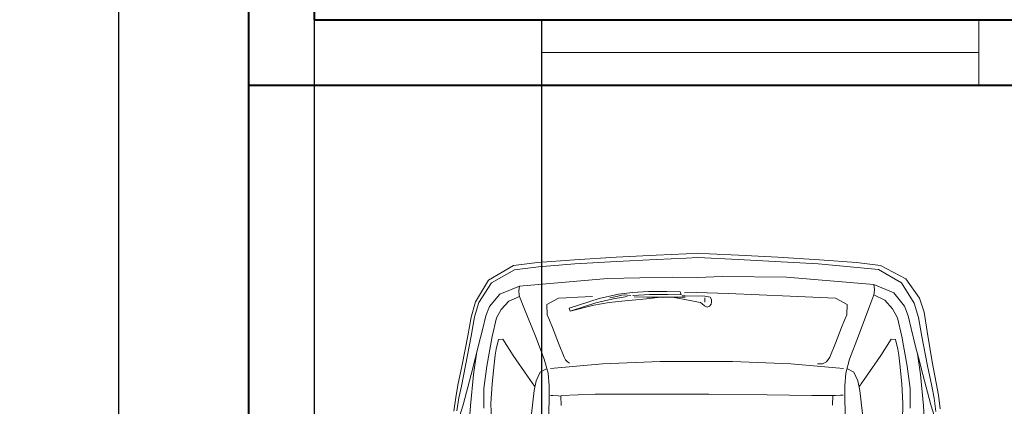
# Model space of a CAD drawing. Units: inches. Extents: x -19 to 419, y -828 to 43.
# Tile 3 of 9: x -9 to 126, y -627 to -574. Entities that reach past the tile are written whole.
import ezdxf

# ---------------------------------------------------------------- set-up
doc = ezdxf.new("R2010")
doc.units = ezdxf.units.IN
doc.header["$MEASUREMENT"] = 0
for name, color, linetype, lineweight in [('A-ANNO-DIMS', 2, 'Continuous', 18), ('A-EQPM-VEHI', 8, 'Continuous', 13), ('A-GLAZ', 4, 'Continuous', 20), ('A-WALL', 7, 'Continuous', 40)]:
    doc.layers.add(name, color=color, linetype=linetype, lineweight=lineweight)
doc.styles.get("Standard").update_dxf_attribs({"font": 'arial.ttf'})
doc.dimstyles.get("Standard").update_dxf_attribs({"dimtxt": 0.18, "dimasz": 0.18, "dimexe": 0.18, "dimexo": 0.0625, "dimgap": 0.09, "dimtad": 0, "dimtih": 1, "dimtoh": 1, "dimdec": 0, "dimzin": 0, "dimdsep": 46, "dimlunit": 3, "dimtxsty": 'Standard', "dimcen": 0.09, "dimadec": 0, "dimazin": 0, "dimtfac": 1, "dimtdec": 0, "dimtofl": 0, "dimtmove": 0, "dimatfit": 3, "dimfxl": 1, "dimtolj": 1, "dimtzin": 0, "dimarcsym": 0})

# ---------------------------------------------------------------- blocks, each defined once
blk = doc.blocks.new('*D2')
at = {"layer": 'A-ANNO-DIMS', "color": 0, "lineweight": -2, "transparency": 16777216}
for p, q in [((22.68, 4.77), (4.74, 4.77)), ((4.92, 4.59), (4.92, -387.33)), ((4.92, -785.55), (4.92, -393.64)), ((22.68, -785.73), (4.74, -785.73))]:
    blk.add_line(p, q, dxfattribs=at)
at = {"layer": 'A-ANNO-DIMS', "color": 0, "transparency": 16777216}
for points in [[(4.89, 4.59), (4.95, 4.59), (4.92, 4.77)], [(4.89, -785.55), (4.95, -785.55), (4.92, -785.73)]]:
    blk.add_solid(points, dxfattribs=at)
at = {"layer": 'Defpoints', "color": 0, "transparency": 16777216}
for p in [(22.74, 4.77), (4.92, -785.73), (22.74, -785.73)]:
    blk.add_point(p, dxfattribs=at)
at = {"layer": 'A-ANNO-DIMS', "color": 0, "transparency": 16777216, "insert": (4.92, -390.48), "char_height": 6, "attachment_point": 5}
blk.add_mtext('\\A1;65\'-11"', dxfattribs=at)
blk = doc.blocks.new('WIN-60X9')
for p, q in [((60, 9), (0, 9)), ((0, 9), (0, 0)), ((60, 0), (60, 9)), ((0, 4.5), (60, 4.5)), ((0, 0), (60, 0))]:
    blk.add_line(p, q)
blk = doc.blocks.new('*D49')
at = {"layer": 'A-ANNO-DIMS', "color": 0, "lineweight": -2, "transparency": 16777216}
for p, q in [((31.74, -574.3), (31.74, -827.51)), ((62.91, -574.3), (62.91, -827.51)), ((31.92, -827.33), (46.99, -827.33)), ((62.73, -827.33), (47.65, -827.33))]:
    blk.add_line(p, q, dxfattribs=at)
at = {"layer": 'A-ANNO-DIMS', "color": 0, "transparency": 16777216}
for points in [[(31.92, -827.3), (31.92, -827.36), (31.74, -827.33)], [(62.73, -827.3), (62.73, -827.36), (62.91, -827.33)]]:
    blk.add_solid(points, dxfattribs=at)
at = {"layer": 'Defpoints', "color": 0, "transparency": 16777216}
for p in [(31.74, -574.23), (62.91, -574.23), (62.91, -827.33)]:
    blk.add_point(p, dxfattribs=at)
at = {"layer": 'A-ANNO-DIMS', "color": 0, "transparency": 16777216, "insert": (47.32, -827.33), "char_height": 0.18, "attachment_point": 5}
blk.add_mtext('\\A1;2\'-7"', dxfattribs=at)

msp = doc.modelspace()

# ---------------------------------------------------------------- linework, layer by layer
at = {"layer": 'A-EQPM-VEHI'}
for p, q in [((73.18, -606.78), (78.63, -606.51)), ((78.63, -606.51), (82.76, -606.33)), ((82.76, -606.33), (84.39, -606.26)), ((84.39, -606.26), (85.95, -606.33)), ((85.95, -606.33), (89.95, -606.51)), ((89.95, -606.51), (95.33, -606.78)), ((59.08, -607.94), (62.39, -607.52)), ((62.39, -607.52), (67.44, -607.13)), ((67.51, -607.72), (62.49, -608.11)), ((67.44, -607.13), (73.18, -606.78)), ((73.21, -607.37), (67.51, -607.72)), ((78.65, -607.1), (73.21, -607.37)), ((82.75, -606.92), (78.65, -607.1)), ((84.37, -606.85), (82.75, -606.92)), ((89.88, -607.09), (84.37, -606.85)), ((100.89, -607.7), (89.88, -607.09)), ((95.33, -606.78), (101.07, -607.13)), ((109.15, -608.49), (100.89, -607.7)), ((101.07, -607.13), (106.12, -607.52)), ((106.12, -607.52), (109.43, -607.94)), ((55.65, -609.93), (59.08, -607.94)), ((59.2, -608.52), (56.05, -610.32)), ((62.49, -608.11), (59.2, -608.52)), ((112.31, -610.32), (109.15, -608.49)), ((109.43, -607.94), (112.9, -609.75)), ((53.85, -612.9), (55.65, -609.93)), ((56.05, -610.32), (54.33, -613.02)), ((59.89, -610.74), (71.96, -609.7)), ((71.96, -609.7), (80.85, -609.51)), ((80.85, -609.51), (84.32, -609.58)), ((84.32, -609.58), (87.73, -609.46)), ((87.73, -609.46), (96.52, -609.55)), ((96.52, -609.55), (108.53, -610.55)), ((111.26, -611.69), (108.53, -610.55)), ((108.59, -611.2), (108.53, -610.55)), ((114.06, -613.09), (112.31, -610.32)), ((112.9, -609.75), (114.79, -612.41)), ((55.79, -613.54), (57.19, -611.84)), ((57.19, -611.84), (59.89, -610.74)), ((59.83, -611.4), (59.89, -610.74)), ((59.86, -611.93), (59.83, -611.4)), ((73.49, -611.87), (70.84, -612.47)), ((75.39, -611.61), (73.49, -611.87)), ((77.61, -611.49), (75.39, -611.61)), ((75.52, -612.04), (77.74, -611.92)), ((80.12, -611.49), (77.61, -611.49)), ((77.74, -611.92), (80.25, -611.92)), ((81.94, -611.55), (80.12, -611.49)), ((80.25, -611.92), (82.07, -611.97)), ((82.07, -611.97), (81.94, -611.55)), ((82.54, -611.69), (84.25, -611.63)), ((84.25, -611.63), (88.54, -611.79)), ((88.54, -611.79), (97.05, -612.12)), ((108.53, -611.96), (108.56, -611.74)), ((108.56, -611.74), (108.59, -611.2)), ((112.7, -613.49), (111.26, -611.69)), ((53.26, -615), (53.85, -612.9)), ((54.33, -613.02), (53.73, -614.97)), ((57.4, -613.94), (58.44, -612.81)), ((58.44, -612.81), (59.89, -612.16)), ((59.89, -612.16), (59.86, -611.93)), ((60.61, -613.93), (59.89, -612.16)), ((63.64, -613.27), (65.24, -612.4)), ((65.24, -612.4), (66.32, -612.34)), ((66.32, -612.34), (67.92, -612.27)), ((70.84, -612.47), (66.71, -613.78)), ((66.84, -614.21), (70.39, -613.07)), ((67.92, -612.27), (69.91, -612.18)), ((70.1, -613.39), (72.22, -613.01)), ((70.39, -613.07), (72.75, -612.5)), ((72.22, -613.01), (73.93, -612.8)), ((72.29, -612.38), (73.23, -612.16)), ((72.75, -612.5), (74.69, -612.16)), ((73.23, -612.16), (73.96, -612.01)), ((73.93, -612.8), (75.37, -612.66)), ((73.96, -612.01), (74.25, -611.96)), ((74.25, -611.96), (75.19, -612.03)), ((75.37, -612.66), (77.32, -612.48)), ((75.44, -612.05), (75.47, -612.05)), ((75.47, -612.05), (75.5, -612.04)), ((75.5, -612.04), (75.52, -612.04)), ((75.65, -612.24), (77.36, -612.25)), ((77.32, -612.48), (79.27, -612.25)), ((77.36, -612.25), (80.62, -612.25)), ((80.62, -612.25), (82.63, -612.26)), ((80.89, -612.25), (83.31, -612.74)), ((82.23, -612.08), (82.61, -612.08)), ((82.61, -612.08), (85.31, -612.15)), ((83.31, -612.74), (84.44, -612.96)), ((84.44, -612.96), (84.73, -613.01)), ((84.96, -613.19), (84.73, -613.01)), ((85.28, -613.48), (84.96, -613.19)), ((85.31, -612.15), (86.07, -612.27)), ((85.35, -612.36), (85.31, -612.94)), ((86.19, -613.22), (85.96, -613.51)), ((86.07, -612.27), (86.24, -612.6)), ((86.25, -612.97), (86.19, -613.22)), ((86.24, -612.6), (86.25, -612.97)), ((97.05, -612.12), (103.27, -612.4)), ((103.27, -612.4), (104.87, -613.27)), ((107.84, -613.78), (108.53, -611.96)), ((110.01, -612.66), (108.53, -611.96)), ((111.08, -613.89), (110.01, -612.66)), ((114.66, -615.07), (114.06, -613.09)), ((114.79, -612.41), (115.42, -614.33)), ((55.28, -614.84), (55.79, -613.54)), ((56.76, -615.1), (57.4, -613.94)), ((62.08, -617.61), (60.61, -613.93)), ((63.69, -614.68), (63.64, -613.27)), ((66.71, -613.78), (66.84, -614.21)), ((66.84, -614.21), (70.1, -613.39)), ((85.63, -613.64), (85.28, -613.48)), ((85.96, -613.51), (85.63, -613.64)), ((104.87, -613.27), (104.81, -614.68)), ((106.4, -617.56), (107.84, -613.78)), ((111.74, -615.1), (111.08, -613.89)), ((113.22, -614.84), (112.7, -613.49)), ((115.42, -614.33), (115.83, -617)), ((52.8, -617.58), (53.26, -615)), ((53.73, -614.97), (53.28, -617.6)), ((54.86, -616.55), (55.28, -614.84)), ((56.14, -617.67), (56.76, -615.1)), ((64.02, -615.42), (63.69, -614.68)), ((64.41, -616.44), (64.02, -615.42)), ((104.49, -615.42), (104.1, -616.44)), ((104.81, -614.68), (104.49, -615.42)), ((112.37, -617.67), (111.74, -615.1)), ((113.65, -616.55), (113.22, -614.84)), ((115.11, -617.67), (114.66, -615.07)), ((54.25, -619.02), (54.86, -616.55)), ((65.24, -618.58), (64.41, -616.44)), ((104.1, -616.44), (103.27, -618.58)), ((114.25, -619.02), (113.65, -616.55)), ((115.83, -617), (116.52, -621.14)), ((52.04, -621.55), (52.8, -617.58)), ((53.28, -617.6), (52.51, -621.65)), ((55.43, -621.71), (56.14, -617.67)), ((56.68, -619.4), (57.02, -618.08)), ((57.02, -618.08), (57.6, -618.05)), ((57.6, -618.05), (59.04, -620.26)), ((63.31, -620.75), (62.08, -617.61)), ((66.01, -620.49), (65.24, -618.58)), ((103.27, -618.58), (102.49, -620.49)), ((105.19, -620.75), (106.4, -617.56)), ((110.91, -618.05), (109.46, -620.26)), ((111.49, -618.08), (110.91, -618.05)), ((111.83, -619.4), (111.49, -618.08)), ((113.07, -621.71), (112.37, -617.67)), ((115.88, -621.67), (115.11, -617.67)), ((53.87, -620.56), (54.25, -619.02)), ((56.57, -620.24), (56.68, -619.4)), ((111.94, -620.24), (111.83, -619.4)), ((114.63, -620.56), (114.25, -619.02)), ((53.28, -622.86), (53.87, -620.56)), ((53.58, -622.89), (54, -620.05)), ((56.43, -621.45), (56.57, -620.24)), ((59.04, -620.26), (60.99, -623.08)), ((63.82, -622.68), (63.31, -620.75)), ((66.22, -620.87), (66.01, -620.49)), ((66.47, -621.14), (66.22, -620.87)), ((66.76, -621.3), (66.47, -621.14)), ((71.31, -621.43), (79.19, -621.08)), ((79.19, -621.08), (84.12, -621.07)), ((84.12, -621.07), (89.13, -621.08)), ((89.13, -621.08), (97.13, -621.43)), ((102.03, -621.14), (101.45, -621.39)), ((102.49, -620.49), (102.03, -621.14)), ((104.68, -622.68), (105.19, -620.75)), ((109.46, -620.26), (107.52, -623.08)), ((112.07, -621.45), (111.94, -620.24)), ((114.93, -622.89), (114.51, -620.05)), ((115.22, -622.86), (114.63, -620.56)), ((116.52, -621.14), (117.06, -624.02)), ((51.46, -624.34), (52.04, -621.55)), ((52.51, -621.65), (51.93, -624.49)), ((55.03, -624.8), (55.43, -621.71)), ((56.17, -624.14), (56.43, -621.45)), ((62.2, -623.72), (62.72, -622.56)), ((62.72, -622.56), (63.7, -622.04)), ((63.96, -624.42), (63.82, -622.68)), ((64.15, -622.04), (71.31, -621.43)), ((97.13, -621.43), (104.36, -622.04)), ((101.45, -621.39), (100.8, -621.4)), ((104.55, -624.42), (104.68, -622.68)), ((105.79, -622.56), (104.81, -622.04)), ((106.31, -623.72), (105.79, -622.56)), ((112.34, -624.14), (112.07, -621.45)), ((113.48, -624.8), (113.07, -621.71)), ((116.47, -624.48), (115.88, -621.67)), ((52.17, -627.01), (53.28, -622.86)), ((53.18, -627.18), (53.58, -622.89)), ((60.99, -623.08), (61.96, -624.48)), ((61.9, -625.06), (62.2, -623.72)), ((106.61, -625.06), (106.31, -623.72)), ((107.52, -623.08), (106.54, -624.48)), ((115.32, -627.18), (114.93, -622.89)), ((116.34, -627.01), (115.22, -622.86)), ((117.06, -624.02), (117.37, -625.69)), ((51.15, -626.02), (51.46, -624.34)), ((51.93, -624.49), (51.59, -626.09)), ((55.01, -627.49), (55.03, -624.8)), ((55.99, -626.85), (56.17, -624.14)), ((61.53, -628.28), (61.9, -625.06)), ((63.96, -626.08), (63.96, -624.42)), ((104.55, -626.08), (104.55, -624.42)), ((106.97, -628.28), (106.61, -625.06)), ((112.51, -626.85), (112.34, -624.14)), ((113.5, -627.49), (113.48, -624.8)), ((116.77, -626.12), (116.47, -624.48)), ((50.91, -627.91), (51.15, -626.02)), ((51.59, -626.09), (51.31, -627.85)), ((63.86, -631.09), (63.96, -626.08)), ((64.49, -625.77), (64.16, -625.75)), ((65.19, -625.8), (64.49, -625.77)), ((65.57, -625.82), (65.19, -625.8)), ((65.61, -627.13), (65.57, -625.82)), ((65.63, -625.76), (70.28, -625.59)), ((70.28, -625.59), (77.53, -625.55)), ((77.53, -625.55), (85.88, -625.59)), ((85.88, -625.59), (93.87, -625.68)), ((93.87, -625.68), (100.03, -625.75)), ((100.03, -625.75), (102.88, -625.76)), ((102.84, -627.08), (102.88, -625.76)), ((102.88, -625.76), (103.26, -625.75)), ((103.26, -625.75), (103.96, -625.71)), ((103.96, -625.71), (104.29, -625.7)), ((104.65, -631.09), (104.55, -626.08)), ((117.01, -627.96), (116.77, -626.12)), ((117.37, -625.69), (117.61, -627.58)), ((51.11, -630.39), (52.17, -627.01)), ((52.97, -630.19), (53.18, -627.18)), ((56.07, -629.23), (55.99, -626.85)), ((112.44, -629.23), (112.51, -626.85)), ((115.53, -630.19), (115.32, -627.18)), ((117.4, -630.39), (116.34, -627.01))]:
    msp.add_line(p, q, dxfattribs=at)
at = {"layer": 'A-WALL'}
for p, q in [((22.74, 4.77), (22.74, -785.73)), ((31.74, -430.23), (31.74, -574.23)), ((31.74, -574.23), (199.74, -574.23)), ((22.74, -583.23), (195.24, -583.23))]:
    msp.add_line(p, q, dxfattribs=at)

# ---------------------------------------------------------------- block references
at = {"layer": 'A-GLAZ'}
msp.add_blockref('WIN-60X9', (62.91, -583.23), dxfattribs=at)

# ---------------------------------------------------------------- dimensions: what is measured, and where the dimension line sits
at = {"layer": 'A-ANNO-DIMS'}
dim = msp.add_linear_dim(base=(4.917623, -785.73343372), p1=(22.73889525, 4.76656628), p2=(22.73889525, -785.73343372), angle=90, dimstyle='Standard', override={"dimtxt": 6, "dimclrd": 0, "dimclre": 0, "dimclrt": 0}, dxfattribs=at)
dim.commit()
dim.dimension.update_dxf_attribs({"geometry": '*D2', "text_midpoint": (4.917623, -390.48343372)})
dim = msp.add_linear_dim(base=(62.91, -827.33), p1=(31.74, -574.23), p2=(62.91, -574.23), dimstyle='Standard', override={"dimdec": 1, "dimlfac": 1, "dimrnd": 0, "dimzin": 1, "dimdsep": 46, "dimlunit": 4, "dimfrac": 2}, dxfattribs=at)
dim.commit()
dim.dimension.update_dxf_attribs({"geometry": '*D49', "text_midpoint": (47.32, -827.33)})

doc.saveas('drawing.dxf')
